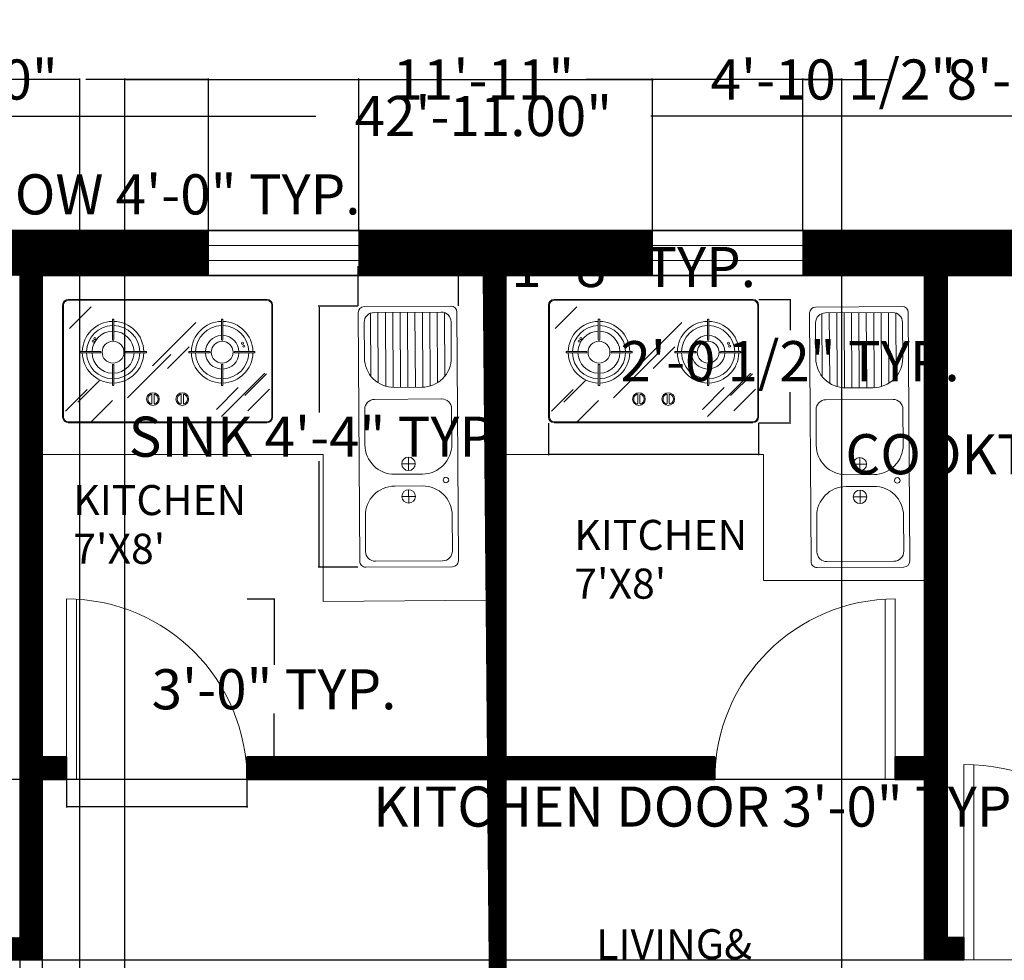
# Model space of a CAD drawing. Units: inches. Extents: x 108 to 771, y 58 to 590.
# Tile 6 of 8: x 327 to 524, y 402 to 590. Entities that reach past the tile are written whole.
import ezdxf

# ---------------------------------------------------------------- set-up
doc = ezdxf.new("R2010")
doc.units = ezdxf.units.IN
doc.header["$MEASUREMENT"] = 0
for name, color, linetype, lineweight in [('A-ANNO-DIMS', 2, 'Continuous', 13), ('A-AREA-IDEN', 7, 'Continuous', 18), ('A-DOOR', 3, 'Continuous', 18), ('A-EQPM', 9, 'Continuous', 15), ('A-FLOR-CASE', 8, 'Continuous', 18), ('A-FLOR-FIXT', 8, 'Continuous', 15), ('A-GLAZ', 4, 'Continuous', 18), ('A-WALL', 7, 'Continuous', 35), ('A-WALL-PATT', 252, 'Continuous', 9)]:
    doc.layers.add(name, color=color, linetype=linetype, lineweight=lineweight)
doc.styles.get("Standard").update_dxf_attribs({"font": 'italic8.shx'})
doc.dimstyles.get("Standard").update_dxf_attribs({"dimtxt": 8, "dimasz": 0.18, "dimexe": 0.18, "dimexo": 0.0625, "dimgap": 0.09, "dimtad": 0, "dimtih": 1, "dimtoh": 1, "dimzin": 0, "dimdsep": 46, "dimlunit": 3, "dimtxsty": 'Standard', "dimcen": 0.09, "dimclrt": 6, "dimadec": 0, "dimazin": 0, "dimtfac": 1, "dimtofl": 0, "dimtmove": 0, "dimatfit": 3, "dimfxl": 1, "dimtolj": 1, "dimtzin": 0, "dimarcsym": 0})

# ---------------------------------------------------------------- blocks, each defined once
blk = doc.blocks.new('*D5')
at = {"layer": 'A-ANNO-DIMS', "color": 0, "lineweight": -2, "transparency": 16777216}
for p, q in [((162.35, 548.12), (162.35, 571.05)), ((162.53, 570.87), (386.42, 570.87)), ((677.17, 570.87), (453.27, 570.87)), ((677.35, 548.12), (677.35, 571.05))]:
    blk.add_line(p, q, dxfattribs=at)
at = {"layer": 'A-ANNO-DIMS', "color": 0, "transparency": 16777216}
for points in [[(162.53, 570.9), (162.53, 570.84), (162.35, 570.87)], [(677.17, 570.9), (677.17, 570.84), (677.35, 570.87)]]:
    blk.add_solid(points, dxfattribs=at)
at = {"layer": 'Defpoints', "color": 0, "transparency": 16777216}
for p in [(677.35, 570.87), (162.35, 548.05), (677.35, 548.05)]:
    blk.add_point(p, dxfattribs=at)
at = {"layer": 'A-ANNO-DIMS', "color": 0, "transparency": 16777216, "insert": (419.85, 570.87), "char_height": 8, "attachment_point": 5}
blk.add_mtext('\\A1;42\'-11.00"', dxfattribs=at)
blk = doc.blocks.new('DOOR-SINGLE-39')
for p, q in [((0, 39), (0, 0)), ((2, 38.95), (2, 0)), ((0, 0), (39, 0))]:
    blk.add_line(p, q)
blk.add_arc((0, 0), 39, 0, 90)
blk = doc.blocks.new('DOOR-SINGLE-36')
for p, q in [((0, 0), (0, 36)), ((2, 0), (2, 35.94)), ((36, 0), (0, 0))]:
    blk.add_line(p, q)
blk.add_arc((0, 0), 36, 0, 90)
blk = doc.blocks.new('WINDOW-30')
for p, q in [((0, 0), (0, 30)), ((0, 30), (9, 30)), ((3, 30), (3, 0)), ((6, 30), (6, 0)), ((9, 30), (9, 0)), ((9, 0), (0, 0))]:
    blk.add_line(p, q)
blk = doc.blocks.new('COOKTOP-TWO-BURNER')
for p, q in [((40.77, 24.58), (1.12, 24.58)), ((40.77, 24.41), (1.12, 24.41)), ((0, 23.46), (0, 1.12)), ((0.17, 23.46), (0.17, 1.12)), ((1.34, 18.81), (5.66, 23.13)), ((41.72, 1.12), (41.72, 23.46)), ((41.89, 1.12), (41.89, 23.46)), ((9.92, 20.64), (10.2, 20.64)), ((9.92, 16.57), (9.92, 20.64)), ((10.2, 16.57), (10.2, 20.64)), ((17.92, 11.32), (26.57, 19.96)), ((31.97, 20.64), (31.69, 20.64)), ((31.69, 16.57), (31.69, 20.64)), ((31.97, 16.57), (31.97, 20.64)), ((7.55, 14.2), (3.53, 14.2)), ((3.53, 14.2), (3.53, 13.92)), ((7.55, 13.92), (3.53, 13.92)), ((12.57, 14.2), (16.7, 14.2)), ((12.57, 13.92), (16.7, 13.92)), ((16.7, 14.2), (16.7, 13.92)), ((20.9, 10.82), (25.22, 15.15)), ((25.19, 14.2), (25.19, 13.92)), ((29.32, 14.2), (25.19, 14.2)), ((29.32, 13.92), (25.19, 13.92)), ((34.34, 14.2), (38.36, 14.2)), ((34.34, 13.92), (38.36, 13.92)), ((38.36, 14.2), (38.36, 13.92)), ((12.96, 4.99), (21.61, 13.63)), ((9.92, 11.55), (9.92, 7.44)), ((10.2, 11.55), (10.2, 7.44)), ((31.69, 11.55), (31.69, 7.44)), ((31.7, 1.24), (40.35, 9.89)), ((31.97, 11.55), (31.97, 7.44)), ((3.04, 4.11), (7.37, 8.43)), ((36.33, 5.43), (40.66, 9.75)), ((0.56, 2.29), (4.89, 6.61)), ((9.92, 7.44), (10.2, 7.44)), ((30.71, 2.67), (35.03, 7)), ((31.97, 7.44), (31.69, 7.44)), ((36.94, 2.34), (41.26, 6.67)), ((5.63, 0.09), (9.96, 4.41)), ((17.8, 5.57), (17.8, 3.86)), ((18.24, 5.57), (18.24, 3.86)), ((23.65, 5.57), (23.65, 3.86)), ((24.09, 5.57), (24.09, 3.86)), ((1.12, 0.17), (40.77, 0.17)), ((1.12, 0), (40.77, 0))]:
    blk.add_line(p, q)
for centre, radius in [((6.11, 16.27), 0.2), ((6.44, 16.77), 0.2), ((10.06, 14.06), 2.18), ((31.83, 14.06), 2.18), ((35.9, 15.84), 0.2), ((36.13, 15.25), 0.2), ((18.02, 4.71), 1.26), ((23.87, 4.71), 1.26)]:
    blk.add_circle(centre, radius)
for centre, radius, start, end in [((1.12, 23.46), 1.12, 90, 180), ((1.12, 23.46), 0.95, 90, 180), ((40.77, 23.46), 1.12, 0, 90), ((40.77, 23.46), 0.95, 0, 90), ((10.06, 14.06), 6.14, 91.3023, 178.6977), ((10.06, 14.06), 6.14, 1.3023, 88.6977), ((31.83, 14.06), 6.14, 91.3023, 178.6977), ((31.83, 14.06), 6.14, 1.3023, 88.6977), ((10.06, 14.06), 5.31, 91.5918, 178.4082), ((10.06, 14.06), 4.19, 91.9102, 178.0898), ((10.06, 14.06), 4.19, 1.9102, 88.0898), ((10.06, 14.06), 5.31, 1.5918, 88.4082), ((31.83, 14.06), 5.31, 91.5918, 178.4082), ((31.83, 14.06), 5.31, 1.5918, 88.4082), ((10.06, 16.59), 0.141, 186.7354, 353.2646), ((31.83, 14.06), 3.35, 92.388, 177.612), ((31.83, 16.58), 0.14, 183.9579, 356.0421), ((31.83, 14.06), 3.35, 2.388, 87.612), ((10.06, 14.06), 6.14, 181.3023, 268.6977), ((10.06, 14.06), 5.31, 181.5918, 268.4082), ((10.06, 14.06), 4.19, 181.9102, 268.0898), ((7.5, 14.06), 0.147, 288.751, 71.249), ((10.06, 14.06), 4.19, 271.9102, 358.0898), ((10.06, 14.06), 6.14, 271.3023, 358.6977), ((10.06, 14.06), 5.31, 271.5918, 358.4082), ((12.62, 14.06), 0.149, 110.5507, 249.4493), ((31.83, 14.06), 6.14, 181.3023, 268.6977), ((31.83, 14.06), 5.31, 181.5918, 268.4082), ((31.83, 14.06), 3.35, 182.388, 267.612), ((29.28, 14.06), 0.147, 288.412, 71.588), ((31.83, 14.06), 3.35, 272.388, 357.612), ((31.83, 14.06), 6.14, 271.3023, 358.6977), ((31.83, 14.06), 5.31, 271.5918, 358.4082), ((34.38, 14.06), 0.144, 104.2945, 255.7055), ((10.06, 11.49), 0.15, 21.7885, 158.2115), ((31.83, 11.51), 0.147, 17.9418, 162.0582), ((18.02, 4.71), 1.03, 111.3237, 248.6763), ((17.69, 5.57), 0.112, 0, 111.3237), ((18.36, 5.57), 0.112, 68.6763, 180), ((18.02, 4.71), 1.03, 291.3237, 68.6763), ((23.87, 4.71), 1.03, 111.3237, 248.6763), ((23.53, 5.57), 0.112, 0, 111.3237), ((24.2, 5.57), 0.112, 68.6763, 180), ((23.87, 4.71), 1.03, 291.3237, 68.6763), ((17.69, 3.86), 0.112, 248.6763, 0), ((18.36, 3.86), 0.112, 180, 291.3237), ((23.53, 3.86), 0.112, 248.6763, 0), ((24.2, 3.86), 0.112, 180, 291.3237), ((1.12, 1.12), 1.12, 180, 270), ((1.12, 1.12), 0.95, 180, 270), ((40.77, 1.12), 0.95, 270, 360), ((40.77, 1.12), 1.12, 270, 360)]:
    blk.add_arc(centre, radius, start, end)
blk = doc.blocks.new('SINK-DOUBLE-DRAINBOARD')
for p, q in [((18.5, 52.07), (1.17, 51.97)), ((0, 50.78), (0.28, 1.17)), ((2.44, 50.65), (2.52, 38.11)), ((16.54, 50.87), (3.15, 50.8)), ((3.92, 50.8), (4, 36.77)), ((5.4, 50.81), (5.48, 36.1)), ((6.87, 50.82), (6.96, 35.86)), ((8.35, 50.83), (8.43, 35.87)), ((9.82, 50.84), (9.91, 35.88)), ((11.3, 50.84), (11.39, 35.88)), ((12.78, 50.85), (12.86, 35.89)), ((14.25, 50.86), (14.34, 36.13)), ((15.73, 50.87), (15.81, 36.8)), ((17.21, 50.77), (17.28, 38.11)), ((19.68, 50.89), (19.97, 1.29)), ((1.23, 41.73), (1.19, 48.82)), ((18.56, 41.83), (18.52, 48.92)), ((12.68, 35.89), (7.17, 35.86)), ((16.63, 33.55), (3.25, 33.48)), ((1.33, 24.41), (1.29, 31.5)), ((18.66, 24.51), (18.61, 31.59)), ((10.02, 19.28), (10.01, 21.96)), ((11.36, 20.63), (8.67, 20.62)), ((12.78, 18.57), (7.27, 18.54)), ((12.8, 16.21), (7.29, 16.18)), ((11.39, 14.13), (8.71, 14.11)), ((10.06, 12.78), (10.05, 15.46)), ((1.41, 10.24), (1.45, 3.15)), ((18.74, 10.34), (18.78, 3.25)), ((18.8, 0.1), (1.47, 0)), ((16.82, 1.27), (3.43, 1.19))]:
    blk.add_line(p, q)
for centre, radius in [((10.02, 20.62), 1.34), ((17.48, 17.39), 0.554), ((10.05, 14.12), 1.34)]:
    blk.add_circle(centre, radius)
for centre, radius, start, end in [((1.18, 50.79), 1.18, 90.3287, 180.3287), ((18.5, 50.89), 1.18, 0.3287, 90.3287), ((3.16, 48.83), 1.97, 90.3287, 180.3287), ((16.55, 48.91), 1.97, 0.3287, 90.3287), ((7.14, 41.77), 5.91, 180.3287, 270.3287), ((12.65, 41.8), 5.91, 270.3287, 0.3287), ((3.26, 31.51), 1.97, 90.3287, 180.3287), ((16.65, 31.58), 1.97, 0.3287, 90.3287), ((7.24, 24.44), 5.91, 180.3287, 270.3287), ((12.75, 24.47), 5.91, 270.3287, 0.3287), ((7.32, 10.27), 5.91, 90.3287, 180.3287), ((12.83, 10.3), 5.91, 0.3287, 90.3287), ((3.42, 3.16), 1.97, 180.3287, 270.3287), ((16.81, 3.24), 1.97, 270.3287, 0.3287), ((1.47, 1.18), 1.18, 180.3287, 270.3287), ((18.79, 1.28), 1.18, 270.3287, 0.3287)]:
    blk.add_arc(centre, radius, start, end)
blk = doc.blocks.new('*D20')
at = {"layer": 'A-ANNO-DIMS', "color": 0, "lineweight": -2, "transparency": 16777216}
for p, q in [((232.77, 548.12), (232.77, 555.43)), ((232.95, 555.25), (280.59, 555.25)), ((280.77, 548.12), (280.77, 555.43)), ((280.77, 555.25), (280.95, 555.25))]:
    blk.add_line(p, q, dxfattribs=at)
at = {"layer": 'A-ANNO-DIMS', "color": 0, "transparency": 16777216}
for points in [[(232.95, 555.28), (232.95, 555.22), (232.77, 555.25)], [(280.59, 555.28), (280.59, 555.22), (280.77, 555.25)]]:
    blk.add_solid(points, dxfattribs=at)
at = {"layer": 'Defpoints', "color": 0, "transparency": 16777216}
for p in [(280.77, 555.25), (232.77, 548.05), (280.77, 548.05)]:
    blk.add_point(p, dxfattribs=at)
at = {"layer": 'A-ANNO-DIMS', "color": 6, "transparency": 16777216, "insert": (346.76, 555.25), "char_height": 8, "attachment_point": 5}
blk.add_mtext('\\A1;WINDOW 4\'-0" TYP.', dxfattribs=at)
blk = doc.blocks.new('*D26')
at = {"layer": 'A-ANNO-DIMS', "color": 0, "lineweight": -2, "transparency": 16777216}
for p, q in [((336.68, 438.49), (336.68, 432.97)), ((372.68, 438.49), (372.68, 432.97)), ((336.86, 433.15), (372.5, 433.15)), ((372.68, 433.15), (372.86, 433.15))]:
    blk.add_line(p, q, dxfattribs=at)
at = {"layer": 'A-ANNO-DIMS', "color": 0, "transparency": 16777216}
for points in [[(336.86, 433.18), (336.86, 433.12), (336.68, 433.15)], [(372.5, 433.18), (372.5, 433.12), (372.68, 433.15)]]:
    blk.add_solid(points, dxfattribs=at)
at = {"layer": 'Defpoints', "color": 0, "transparency": 16777216}
for p in [(336.68, 438.55), (372.68, 438.55), (372.68, 433.15)]:
    blk.add_point(p, dxfattribs=at)
at = {"layer": 'A-ANNO-DIMS', "color": 6, "transparency": 16777216, "insert": (463.04, 433.15), "char_height": 8, "attachment_point": 5}
blk.add_mtext('\\A1;KITCHEN DOOR 3\'-0" TYP.', dxfattribs=at)
blk = doc.blocks.new('*D27')
at = {"layer": 'A-ANNO-DIMS', "color": 0, "lineweight": -2, "transparency": 16777216}
for p, q in [((372.74, 474.55), (378.26, 474.55)), ((378.08, 474.37), (378.08, 461.41)), ((378.08, 438.73), (378.08, 451.7)), ((372.74, 438.55), (378.26, 438.55))]:
    blk.add_line(p, q, dxfattribs=at)
at = {"layer": 'A-ANNO-DIMS', "color": 0, "transparency": 16777216}
for points in [[(378.05, 474.37), (378.11, 474.37), (378.08, 474.55)], [(378.05, 438.73), (378.11, 438.73), (378.08, 438.55)]]:
    blk.add_solid(points, dxfattribs=at)
at = {"layer": 'Defpoints', "color": 0, "transparency": 16777216}
for p in [(372.68, 474.55), (378.08, 474.55), (372.68, 438.55)]:
    blk.add_point(p, dxfattribs=at)
at = {"layer": 'A-ANNO-DIMS', "color": 6, "transparency": 16777216, "insert": (378.08, 456.55), "char_height": 8, "attachment_point": 5}
blk.add_mtext('\\A1;3\'-0" TYP.', dxfattribs=at)
blk = doc.blocks.new('*D38')
at = {"layer": 'A-ANNO-DIMS', "color": 0, "lineweight": -2, "transparency": 16777216}
for p, q in [((606.93, 385.95), (606.93, 394.93)), ((665.98, 385.95), (665.98, 394.93)), ((606.93, 394.75), (606.75, 394.75)), ((665.8, 394.75), (607.11, 394.75))]:
    blk.add_line(p, q, dxfattribs=at)
at = {"layer": 'A-ANNO-DIMS', "color": 0, "transparency": 16777216}
for points in [[(607.11, 394.78), (607.11, 394.72), (606.93, 394.75)], [(665.8, 394.78), (665.8, 394.72), (665.98, 394.75)]]:
    blk.add_solid(points, dxfattribs=at)
at = {"layer": 'Defpoints', "color": 0, "transparency": 16777216}
for p in [(606.93, 394.75), (606.93, 385.89), (665.98, 385.89)]:
    blk.add_point(p, dxfattribs=at)
at = {"layer": 'A-ANNO-DIMS', "color": 6, "transparency": 16777216, "insert": (552.56, 394.75), "char_height": 8, "attachment_point": 5}
blk.add_mtext('\\A1;TUB 4\'-11" TYP.', dxfattribs=at)
blk = doc.blocks.new('*D40')
at = {"layer": 'A-ANNO-DIMS', "color": 0, "lineweight": -2, "transparency": 16777216}
for p, q in [((432.85, 509.64), (432.85, 503.24)), ((474.74, 509.64), (474.74, 503.24)), ((433.03, 503.42), (474.56, 503.42)), ((474.74, 503.42), (474.92, 503.42))]:
    blk.add_line(p, q, dxfattribs=at)
at = {"layer": 'A-ANNO-DIMS', "color": 0, "transparency": 16777216}
for points in [[(433.03, 503.45), (433.03, 503.39), (432.85, 503.42)], [(474.56, 503.45), (474.56, 503.39), (474.74, 503.42)]]:
    blk.add_solid(points, dxfattribs=at)
at = {"layer": 'Defpoints', "color": 0, "transparency": 16777216}
for p in [(432.85, 509.7), (474.74, 509.7), (474.74, 503.42)]:
    blk.add_point(p, dxfattribs=at)
at = {"layer": 'A-ANNO-DIMS', "color": 6, "transparency": 16777216, "insert": (543.58, 503.42), "char_height": 8, "attachment_point": 5}
blk.add_mtext('\\A1;COOKTOP 3\'-6" TYP.', dxfattribs=at)
blk = doc.blocks.new('*D41')
at = {"layer": 'A-ANNO-DIMS', "color": 0, "lineweight": -2, "transparency": 16777216}
for p, q in [((474.8, 534.28), (481.2, 534.28)), ((481.02, 534.1), (481.02, 528.18)), ((481.02, 509.88), (481.02, 515.81)), ((474.8, 509.7), (481.2, 509.7))]:
    blk.add_line(p, q, dxfattribs=at)
at = {"layer": 'A-ANNO-DIMS', "color": 0, "transparency": 16777216}
for points in [[(480.99, 534.1), (481.05, 534.1), (481.02, 534.28)], [(480.99, 509.88), (481.05, 509.88), (481.02, 509.7)]]:
    blk.add_solid(points, dxfattribs=at)
at = {"layer": 'Defpoints', "color": 0, "transparency": 16777216}
for p in [(474.74, 534.28), (481.02, 534.28), (474.74, 509.7)]:
    blk.add_point(p, dxfattribs=at)
at = {"layer": 'A-ANNO-DIMS', "color": 6, "transparency": 16777216, "insert": (481.02, 521.99), "char_height": 8, "attachment_point": 5}
blk.add_mtext('\\A1;2\'-0 1/2" TYP.', dxfattribs=at)
blk = doc.blocks.new('*D42')
at = {"layer": 'A-ANNO-DIMS', "color": 0, "lineweight": -2, "transparency": 16777216}
for p, q in [((394.82, 532.96), (386.89, 532.96)), ((387.07, 532.78), (387.07, 511.77)), ((387.07, 481.07), (387.07, 502.07)), ((394.82, 480.89), (386.89, 480.89))]:
    blk.add_line(p, q, dxfattribs=at)
at = {"layer": 'A-ANNO-DIMS', "color": 0, "transparency": 16777216}
for points in [[(387.04, 532.78), (387.1, 532.78), (387.07, 532.96)], [(387.04, 481.07), (387.1, 481.07), (387.07, 480.89)]]:
    blk.add_solid(points, dxfattribs=at)
at = {"layer": 'Defpoints', "color": 0, "transparency": 16777216}
for p in [(387.07, 532.96), (394.88, 532.96), (394.88, 480.89)]:
    blk.add_point(p, dxfattribs=at)
at = {"layer": 'A-ANNO-DIMS', "color": 6, "transparency": 16777216, "insert": (387.07, 506.92), "char_height": 8, "attachment_point": 5}
blk.add_mtext('\\A1;SINK 4\'-4" TYP.', dxfattribs=at)
blk = doc.blocks.new('*D43')
at = {"layer": 'A-ANNO-DIMS', "color": 0, "lineweight": -2, "transparency": 16777216}
for p, q in [((394.88, 533.02), (394.88, 540.95)), ((395.06, 540.77), (414.68, 540.77)), ((414.86, 533.02), (414.86, 540.95)), ((414.86, 540.77), (415.04, 540.77))]:
    blk.add_line(p, q, dxfattribs=at)
at = {"layer": 'A-ANNO-DIMS', "color": 0, "transparency": 16777216}
for points in [[(395.06, 540.8), (395.06, 540.74), (394.88, 540.77)], [(414.68, 540.8), (414.68, 540.74), (414.86, 540.77)]]:
    blk.add_solid(points, dxfattribs=at)
at = {"layer": 'Defpoints', "color": 0, "transparency": 16777216}
for p in [(414.86, 540.77), (394.88, 532.96), (414.86, 532.96)]:
    blk.add_point(p, dxfattribs=at)
at = {"layer": 'A-ANNO-DIMS', "color": 6, "transparency": 16777216, "insert": (449.8, 540.77), "char_height": 8, "attachment_point": 5}
blk.add_mtext('\\A1;1\'-8" TYP.', dxfattribs=at)
blk = doc.blocks.new('*D52')
at = {"layer": 'A-ANNO-DIMS', "color": 0, "lineweight": -2, "transparency": 16777216}
for p, q in [((348.35, 145.12), (348.35, 578.33)), ((348.53, 578.15), (399.37, 578.15)), ((491.17, 578.15), (440.32, 578.15)), ((491.35, 145.12), (491.35, 578.33))]:
    blk.add_line(p, q, dxfattribs=at)
at = {"layer": 'A-ANNO-DIMS', "color": 0, "transparency": 16777216}
for points in [[(348.53, 578.18), (348.53, 578.12), (348.35, 578.15)], [(491.17, 578.18), (491.17, 578.12), (491.35, 578.15)]]:
    blk.add_solid(points, dxfattribs=at)
at = {"layer": 'Defpoints', "color": 0, "transparency": 16777216}
for p in [(491.35, 578.15), (348.35, 145.05), (491.35, 145.05)]:
    blk.add_point(p, dxfattribs=at)
at = {"layer": 'A-ANNO-DIMS', "color": 6, "transparency": 16777216, "insert": (419.85, 578.15), "char_height": 8, "attachment_point": 5}
blk.add_mtext('\\A1;11\'-11"', dxfattribs=at)
blk = doc.blocks.new('*D54')
at = {"layer": 'A-ANNO-DIMS', "color": 0, "lineweight": -2, "transparency": 16777216}
for p, q in [((280.77, 548.12), (280.77, 578.33)), ((280.95, 578.15), (305.28, 578.15)), ((364.84, 578.15), (340.51, 578.15)), ((365.02, 548.12), (365.02, 578.33))]:
    blk.add_line(p, q, dxfattribs=at)
at = {"layer": 'A-ANNO-DIMS', "color": 0, "transparency": 16777216}
for points in [[(280.95, 578.18), (280.95, 578.12), (280.77, 578.15)], [(364.84, 578.18), (364.84, 578.12), (365.02, 578.15)]]:
    blk.add_solid(points, dxfattribs=at)
at = {"layer": 'Defpoints', "color": 0, "transparency": 16777216}
for p in [(365.02, 578.15), (280.77, 548.05), (365.02, 548.05)]:
    blk.add_point(p, dxfattribs=at)
at = {"layer": 'A-ANNO-DIMS', "color": 6, "transparency": 16777216, "insert": (322.9, 578.15), "char_height": 8, "attachment_point": 5}
blk.add_mtext('\\A1;7\'-0"', dxfattribs=at)
blk = doc.blocks.new('*D55')
at = {"layer": 'A-ANNO-DIMS', "color": 0, "lineweight": -2, "transparency": 16777216}
for p, q in [((395.02, 548.12), (395.02, 578.33)), ((395.2, 578.15), (453.4, 578.15)), ((453.58, 548.12), (453.58, 578.33)), ((453.58, 578.15), (453.76, 578.15))]:
    blk.add_line(p, q, dxfattribs=at)
at = {"layer": 'A-ANNO-DIMS', "color": 0, "transparency": 16777216}
for points in [[(395.2, 578.18), (395.2, 578.12), (395.02, 578.15)], [(453.4, 578.18), (453.4, 578.12), (453.58, 578.15)]]:
    blk.add_solid(points, dxfattribs=at)
at = {"layer": 'Defpoints', "color": 0, "transparency": 16777216}
for p in [(453.58, 578.15), (395.02, 548.05), (453.58, 548.05)]:
    blk.add_point(p, dxfattribs=at)
at = {"layer": 'A-ANNO-DIMS', "color": 6, "transparency": 16777216, "insert": (489.66, 578.15), "char_height": 8, "attachment_point": 5}
blk.add_mtext('\\A1;4\'-10 1/2"', dxfattribs=at)
blk = doc.blocks.new('*D56')
at = {"layer": 'A-ANNO-DIMS', "color": 0, "lineweight": -2, "transparency": 16777216}
for p, q in [((483.58, 548.12), (483.58, 578.33)), ((483.76, 578.15), (500.52, 578.15)), ((583.74, 578.15), (566.98, 578.15)), ((583.92, 548.12), (583.92, 578.33))]:
    blk.add_line(p, q, dxfattribs=at)
at = {"layer": 'A-ANNO-DIMS', "color": 0, "transparency": 16777216}
for points in [[(483.76, 578.18), (483.76, 578.12), (483.58, 578.15)], [(583.74, 578.18), (583.74, 578.12), (583.92, 578.15)]]:
    blk.add_solid(points, dxfattribs=at)
at = {"layer": 'Defpoints', "color": 0, "transparency": 16777216}
for p in [(583.92, 578.15), (483.58, 548.05), (583.92, 548.05)]:
    blk.add_point(p, dxfattribs=at)
at = {"layer": 'A-ANNO-DIMS', "color": 6, "transparency": 16777216, "insert": (533.75, 578.15), "char_height": 8, "attachment_point": 5}
blk.add_mtext('\\A1;8\'-4 1/2"', dxfattribs=at)
blk = doc.blocks.new('*D59')
at = {"layer": 'A-ANNO-DIMS', "color": 0, "lineweight": -2, "transparency": 16777216}
for p, q in [((327.35, 538.99), (327.35, 69.77)), ((331.85, 538.99), (331.85, 69.77)), ((327.53, 69.95), (331.67, 69.95)), ((331.85, 69.95), (332.03, 69.95))]:
    blk.add_line(p, q, dxfattribs=at)
at = {"layer": 'A-ANNO-DIMS', "color": 0, "transparency": 16777216}
for points in [[(327.53, 69.98), (327.53, 69.92), (327.35, 69.95)], [(331.67, 69.98), (331.67, 69.92), (331.85, 69.95)]]:
    blk.add_solid(points, dxfattribs=at)
at = {"layer": 'Defpoints', "color": 0, "transparency": 16777216}
for p in [(327.35, 539.05), (331.85, 539.05), (331.85, 69.95)]:
    blk.add_point(p, dxfattribs=at)
at = {"layer": 'A-ANNO-DIMS', "color": 6, "transparency": 16777216, "insert": (365.26, 69.95), "char_height": 8, "attachment_point": 5}
blk.add_mtext('\\A1;0\'-4 1/2"', dxfattribs=at)
blk = doc.blocks.new('*D60')
at = {"layer": 'A-ANNO-DIMS', "color": 0, "lineweight": -2, "transparency": 16777216}
for p, q in [((171.35, 145.12), (171.35, 578.33)), ((171.53, 578.15), (234.87, 578.15)), ((339.17, 578.15), (275.82, 578.15)), ((339.35, 145.12), (339.35, 578.33))]:
    blk.add_line(p, q, dxfattribs=at)
at = {"layer": 'A-ANNO-DIMS', "color": 0, "transparency": 16777216}
for points in [[(171.53, 578.18), (171.53, 578.12), (171.35, 578.15)], [(339.17, 578.18), (339.17, 578.12), (339.35, 578.15)]]:
    blk.add_solid(points, dxfattribs=at)
at = {"layer": 'Defpoints', "color": 0, "transparency": 16777216}
for p in [(339.35, 578.15), (171.35, 145.05), (339.35, 145.05)]:
    blk.add_point(p, dxfattribs=at)
at = {"layer": 'A-ANNO-DIMS', "color": 6, "transparency": 16777216, "insert": (255.35, 578.15), "char_height": 8, "attachment_point": 5}
blk.add_mtext('\\A1;14\'-0"', dxfattribs=at)
blk = doc.blocks.new('*D62')
at = {"layer": 'A-ANNO-DIMS', "color": 0, "lineweight": -2, "transparency": 16777216}
for p, q in [((507.78, 438.55), (132.07, 438.55)), ((132.25, 438.37), (132.25, 425.4)), ((132.25, 402.73), (132.25, 415.7)), ((515.6, 402.55), (132.07, 402.55))]:
    blk.add_line(p, q, dxfattribs=at)
at = {"layer": 'A-ANNO-DIMS', "color": 0, "transparency": 16777216}
for points in [[(132.22, 438.37), (132.28, 438.37), (132.25, 438.55)], [(132.22, 402.73), (132.28, 402.73), (132.25, 402.55)]]:
    blk.add_solid(points, dxfattribs=at)
at = {"layer": 'Defpoints', "color": 0, "transparency": 16777216}
for p in [(507.85, 438.55), (132.25, 402.55), (515.66, 402.55)]:
    blk.add_point(p, dxfattribs=at)
at = {"layer": 'A-ANNO-DIMS', "color": 6, "transparency": 16777216, "insert": (132.25, 420.55), "char_height": 8, "attachment_point": 5}
blk.add_mtext('\\A1;3\'-0"', dxfattribs=at)

msp = doc.modelspace()

# ---------------------------------------------------------------- hatches: boundary and pattern name
at = {"layer": 'A-WALL-PATT'}
h = msp.add_hatch(dxfattribs=at)
h.set_pattern_fill('ANSI31', color=256)
h.paths.add_polyline_path([(171.345, 461.548), (162.345, 461.548), (162.345, 390.901), (171.345, 390.901), (171.345, 393.51), (171.345, 402.553), (233.142, 402.553), (233.142, 407.053), (171.345, 407.053)])
h.paths.add_polyline_path([(331.845, 438.553), (336.68, 438.554), (336.68, 443.053), (331.845, 443.053), (331.845, 539.053), (365.02, 539.053), (365.02, 548.053), (280.772, 548.053), (280.772, 539.053), (327.345, 539.053), (327.345, 407.053), (325.63, 407.053), (325.63, 402.553), (331.845, 402.553)])
h.paths.add_polyline_path([(286.63, 407.053), (263.142, 407.053), (263.142, 402.553), (267.345, 402.553), (267.345, 352.303), (171.345, 352.303), (171.345, 360.901), (162.345, 360.901), (162.345, 336.026), (171.345, 336.026), (171.345, 347.803), (267.345, 347.803), (267.345, 293.053), (263.142, 293.053), (263.142, 288.553), (293.037, 288.553), (293.037, 293.053), (271.845, 293.053), (271.845, 402.553), (286.63, 402.553)])
h.paths.add_polyline_path([(466.018, 443.053), (424.345, 443.053), (424.345, 539.053), (453.584, 539.053), (453.584, 548.053), (395.02, 548.053), (395.02, 539.053), (419.845, 539.053), (420.71, 443.053), (372.68, 443.053), (372.68, 438.557), (420.751, 438.561), (421.075, 402.553), (422.061, 293.053), (419.994, 293.053), (419.994, 288.553), (426.124, 288.553), (426.124, 293.053), (424.345, 293.053), (424.345, 402.553), (424.345, 438.553), (466.018, 438.553)])
h.paths.add_polyline_path([(512.345, 539.053), (583.918, 539.053), (583.918, 548.053), (483.584, 548.053), (483.584, 539.053), (507.845, 539.053), (507.845, 443.053), (502.018, 443.053), (502.018, 438.553), (507.845, 438.553), (507.845, 402.553), (515.658, 402.553), (515.658, 407.053), (512.345, 407.053)])
h.paths.add_polyline_path([(232.772, 548.053), (162.345, 548.053), (162.345, 509.548), (171.345, 509.548), (171.345, 539.053), (232.772, 539.053)])
h.paths.add_polyline_path([(233.142, 293.053), (171.345, 293.053), (171.345, 306.026), (162.345, 306.026), (162.345, 230.8), (171.345, 230.8), (171.345, 288.553), (233.142, 288.553)])
h.paths.add_polyline_path([(359.994, 293.053), (332.037, 293.053), (332.037, 288.553), (339.345, 288.553), (339.345, 145.053), (334.469, 145.053), (334.469, 136.053), (339.345, 136.053), (339.345, 104.553), (166.845, 104.553), (166.845, 136.053), (211.837, 136.053), (211.837, 145.053), (171.345, 145.053), (171.345, 182.8), (162.345, 182.8), (162.345, 100.053), (343.845, 100.053), (343.845, 136.053), (400.886, 136.053), (400.886, 145.053), (348.345, 145.053), (348.345, 288.553), (359.994, 288.553)])
h.paths.add_polyline_path([(500.345, 288.553), (503.755, 288.553), (503.755, 293.053), (486.124, 293.053), (486.124, 288.553), (491.345, 288.553), (491.345, 145.053), (448.886, 145.053), (448.886, 136.053), (495.845, 136.053), (495.845, 100.053), (677.345, 100.053), (677.345, 186.265), (668.345, 186.265), (668.345, 145.053), (627.637, 145.053), (627.637, 136.053), (672.845, 136.053), (672.845, 104.278), (500.345, 104.539), (500.345, 136.053), (504.239, 136.053), (504.239, 145.053), (500.345, 145.053)])
h.paths.add_polyline_path([(580.913, 293.053), (572.345, 293.053), (572.345, 347.803), (668.345, 347.803), (668.345, 330.831), (677.345, 330.831), (677.345, 366.853), (668.345, 366.853), (668.345, 352.303), (572.345, 352.303), (572.345, 402.553), (580.418, 402.553), (580.418, 407.053), (554.658, 407.053), (554.658, 402.553), (567.845, 402.553), (567.845, 293.053), (542.755, 293.053), (542.755, 288.553), (580.913, 288.553)])
h.paths.add_polyline_path([(677.345, 300.831), (668.345, 300.831), (668.345, 293.053), (610.913, 293.053), (610.913, 288.553), (668.345, 288.553), (668.345, 234.265), (677.345, 234.265)])
h.paths.add_polyline_path([(304.469, 145.053), (259.837, 145.053), (259.837, 136.053), (304.469, 136.053)], flags=17)
h.paths.add_polyline_path([(579.637, 145.053), (534.239, 145.053), (534.239, 136.053), (579.637, 136.053)], flags=17)
h.paths.add_polyline_path([(677.345, 450.416), (668.345, 450.416), (668.345, 407.053), (610.418, 407.053), (610.418, 402.553), (668.345, 402.553), (668.345, 396.853), (677.345, 396.853)])
h.paths.add_polyline_path([(677.345, 548.053), (631.918, 548.053), (631.918, 539.053), (668.345, 539.053), (668.345, 498.416), (677.345, 498.416)])
h = msp.add_hatch(dxfattribs=at)
h.set_pattern_fill('ANSI31', color=256)
h.paths.add_polyline_path([(365.02, 548.053), (280.772, 548.053), (280.772, 539.053), (327.345, 539.053), (327.345, 407.053), (325.63, 407.053), (325.63, 402.553), (331.845, 402.553), (331.845, 438.553), (336.68, 438.554), (336.68, 443.053), (331.845, 443.053), (331.845, 539.053), (365.02, 539.053)])
h.paths.add_polyline_path([(453.584, 548.053), (395.02, 548.053), (395.02, 539.053), (419.845, 539.053), (420.71, 443.053), (372.68, 443.053), (372.68, 438.557), (420.751, 438.561), (421.075, 402.553), (422.061, 293.053), (419.994, 293.053), (419.994, 288.553), (426.124, 288.553), (426.124, 293.053), (424.345, 293.053), (424.345, 402.553), (424.345, 438.553), (466.018, 438.553), (466.018, 443.053), (424.345, 443.053), (424.345, 539.053), (453.584, 539.053)])
h.paths.add_polyline_path([(232.772, 548.053), (162.345, 548.053), (162.345, 509.548), (171.345, 509.548), (171.345, 539.053), (232.772, 539.053)])
h.paths.add_polyline_path([(171.345, 461.548), (162.345, 461.548), (162.345, 390.901), (171.345, 390.901), (171.345, 393.51), (171.345, 402.553), (233.142, 402.553), (233.142, 407.053), (171.345, 407.053)])
h.paths.add_polyline_path([(286.63, 407.053), (263.142, 407.053), (263.142, 402.553), (267.345, 402.553), (267.345, 352.303), (171.345, 352.303), (171.345, 360.901), (162.345, 360.901), (162.345, 336.026), (171.345, 336.026), (171.345, 347.803), (267.345, 347.803), (267.345, 293.053), (263.142, 293.053), (263.142, 288.553), (293.037, 288.553), (293.037, 293.053), (271.845, 293.053), (271.845, 402.553), (286.63, 402.553)])
h.paths.add_polyline_path([(171.345, 306.026), (162.345, 306.026), (162.345, 230.8), (171.345, 230.8), (171.345, 288.553), (233.142, 288.553), (233.142, 293.053), (171.345, 293.053)])
h.paths.add_polyline_path([(348.345, 288.553), (359.994, 288.553), (359.994, 293.053), (332.037, 293.053), (332.037, 288.553), (339.345, 288.553), (339.345, 145.053), (334.469, 145.053), (334.469, 136.053), (339.345, 136.053), (339.345, 104.553), (166.845, 104.553), (166.845, 136.053), (211.837, 136.053), (211.837, 145.053), (171.345, 145.053), (171.345, 182.8), (162.345, 182.8), (162.345, 100.053), (343.845, 100.053), (343.845, 136.053), (400.886, 136.053), (400.886, 145.053), (348.345, 145.053)])
h.paths.add_polyline_path([(503.755, 293.053), (486.124, 293.053), (486.124, 288.553), (491.345, 288.553), (491.345, 145.053), (448.886, 145.053), (448.886, 136.053), (495.845, 136.053), (495.845, 100.053), (677.345, 100.053), (677.345, 186.265), (668.345, 186.265), (668.345, 145.053), (627.637, 145.053), (627.637, 136.053), (672.845, 136.053), (672.845, 104.278), (500.345, 104.539), (500.345, 136.053), (504.239, 136.053), (504.239, 145.053), (500.345, 145.053), (500.345, 288.553), (503.755, 288.553)])
h.paths.add_polyline_path([(580.913, 293.053), (572.345, 293.053), (572.345, 347.803), (668.345, 347.803), (668.345, 330.831), (677.345, 330.831), (677.345, 366.853), (668.345, 366.853), (668.345, 352.303), (572.345, 352.303), (572.345, 402.553), (580.418, 402.553), (580.418, 407.053), (554.658, 407.053), (554.658, 402.553), (567.845, 402.553), (567.845, 293.053), (542.755, 293.053), (542.755, 288.553), (580.913, 288.553)])
h.paths.add_polyline_path([(677.345, 300.831), (668.345, 300.831), (668.345, 293.053), (610.913, 293.053), (610.913, 288.553), (668.345, 288.553), (668.345, 234.265), (677.345, 234.265)])
h.paths.add_polyline_path([(579.637, 145.053), (534.239, 145.053), (534.239, 136.053), (579.637, 136.053)], flags=17)
h.paths.add_polyline_path([(304.469, 145.053), (259.837, 145.053), (259.837, 136.053), (304.469, 136.053)], flags=17)
h.paths.add_polyline_path([(583.918, 548.053), (483.584, 548.053), (483.584, 539.053), (507.845, 539.053), (507.845, 443.053), (502.018, 443.053), (502.018, 438.553), (507.845, 438.553), (507.845, 402.553), (515.658, 402.553), (515.658, 407.053), (512.345, 407.053), (512.345, 539.053), (583.918, 539.053)])
h.paths.add_polyline_path([(677.345, 548.053), (631.918, 548.053), (631.918, 539.053), (668.345, 539.053), (668.345, 498.416), (677.345, 498.416)])
h.paths.add_polyline_path([(677.345, 450.416), (668.345, 450.416), (668.345, 407.053), (610.418, 407.053), (610.418, 402.553), (668.345, 402.553), (668.345, 396.853), (677.345, 396.853)])

# ---------------------------------------------------------------- linework, layer by layer
at = {"layer": 'A-FLOR-CASE'}
for p, q in [((331.845, 503.364), (387.855, 503.364)), ((387.855, 503.364), (387.855, 474.038)), ((424.345, 503.364), (475.728, 503.364)), ((475.728, 503.364), (475.728, 478.253)), ((475.728, 478.253), (507.845, 478.253)), ((387.855, 474.038), (420.428, 474.332))]:
    msp.add_line(p, q, dxfattribs=at)
at = {"layer": 'A-WALL'}
for p, q in [((162.345, 548.053), (677.345, 548.053)), ((331.845, 539.053), (419.845, 539.053)), ((331.845, 443.053), (331.845, 539.053)), ((420.71, 443.053), (419.845, 539.053)), ((424.345, 539.053), (507.845, 539.053)), ((424.345, 443.053), (424.345, 539.053)), ((507.845, 539.053), (507.845, 443.053)), ((512.345, 539.053), (512.345, 407.053)), ((512.345, 539.053), (668.345, 539.053)), ((331.845, 443.053), (336.68, 443.053)), ((336.68, 438.554), (336.68, 443.053)), ((372.68, 438.554), (372.68, 443.053)), ((372.68, 443.053), (420.71, 443.053)), ((424.345, 443.053), (466.018, 443.053)), ((466.018, 438.553), (466.018, 443.053)), ((502.018, 438.553), (502.018, 443.053)), ((502.018, 443.053), (507.845, 443.053)), ((331.845, 438.553), (336.68, 438.554)), ((331.845, 402.553), (331.845, 438.553)), ((372.68, 438.557), (420.751, 438.561)), ((421.075, 402.553), (420.751, 438.561)), ((424.345, 402.553), (424.345, 438.553)), ((424.345, 438.553), (466.018, 438.553)), ((502.018, 438.553), (507.845, 438.553)), ((507.845, 438.553), (507.845, 402.553)), ((512.345, 407.053), (515.658, 407.053)), ((515.658, 407.053), (515.658, 402.553)), ((325.63, 402.553), (331.845, 402.553)), ((422.061, 293.053), (421.075, 402.553)), ((424.345, 293.053), (424.345, 402.553)), ((507.845, 402.553), (515.658, 402.553))]:
    msp.add_line(p, q, dxfattribs=at)

# ---------------------------------------------------------------- block references
at = {"layer": 'A-DOOR'}
for name, p in [('DOOR-SINGLE-36', (336.68, 438.554)), ('DOOR-SINGLE-39', (515.658, 402.553))]:
    msp.add_blockref(name, p, dxfattribs=at)
at = {"layer": 'A-DOOR', "extrusion": (0, 0, -1), "zscale": -1}
msp.add_blockref('DOOR-SINGLE-36', (-502.017, 438.554), dxfattribs=at)
at = {"layer": 'A-EQPM'}
for p in [(335.911, 509.705), (432.846, 509.705)]:
    msp.add_blockref('COOKTOP-TWO-BURNER', p, dxfattribs=at)
at = {"layer": 'A-FLOR-FIXT'}
for p in [(394.888, 480.888), (484.932, 480.805)]:
    msp.add_blockref('SINK-DOUBLE-DRAINBOARD', p, dxfattribs=at)
at = {"layer": 'A-GLAZ', "rotation": 90.00000000000006}
for p in [(395.02, 539.053), (483.584, 539.053)]:
    msp.add_blockref('WINDOW-30', p, dxfattribs=at)

# ---------------------------------------------------------------- texts
at = {"layer": 'A-AREA-IDEN'}
for s, p in [('KITCHEN', (338.037, 491.279)), ('KITCHEN', (437.987, 484.327)), ("7'X8'", (338.037, 481.565)), ("7'X8'", (437.987, 474.612)), ('LIVING&', (442.356, 402.701))]:
    msp.add_text(s, height=6, dxfattribs=at).set_placement(p)

# ---------------------------------------------------------------- dimensions: what is measured, and where the dimension line sits
at = {"layer": 'A-ANNO-DIMS'}
for base, p1, p2, override, picture, middle in [((453.584, 578.153), (395.02, 548.053), (453.584, 548.053), {"dimdec": 1, "dimlfac": 1, "dimrnd": 0, "dimzin": 1, "dimdsep": 46, "dimlunit": 4, "dimfrac": 2}, '*D55', (489.664, 578.153)), ((583.918, 578.153), (483.584, 548.053), (583.918, 548.053), {"dimdec": 1, "dimlfac": 1, "dimrnd": 0, "dimzin": 1, "dimdsep": 46, "dimlunit": 4, "dimfrac": 2}, '*D56', (533.751, 578.153)), ((339.345, 578.153), (171.345, 145.053), (339.345, 145.053), {"dimdec": 1, "dimlfac": 1, "dimrnd": 0, "dimzin": 1, "dimdsep": 46, "dimlunit": 4, "dimfrac": 2}, '*D60', (255.345, 578.153)), ((365.02, 578.153), (280.772, 548.053), (365.02, 548.053), {"dimdec": 1, "dimlfac": 1, "dimrnd": 0, "dimzin": 1, "dimdsep": 46, "dimlunit": 4, "dimfrac": 2}, '*D54', (322.896, 578.153)), ((491.345, 578.153), (348.345, 145.053), (491.345, 145.053), {"dimdec": 1, "dimlfac": 1, "dimrnd": 0, "dimzin": 1, "dimdsep": 46, "dimlunit": 4, "dimfrac": 2}, '*D52', (419.845, 578.153)), ((677.345, 570.871), (162.345, 548.053), (677.345, 548.053), {"dimclrd": 0, "dimclre": 0, "dimclrt": 0}, '*D5', (419.845, 570.871)), ((331.845, 69.953), (327.345, 539.053), (331.845, 539.053), {"dimdec": 1, "dimlfac": 1, "dimrnd": 0, "dimzin": 1, "dimdsep": 46, "dimlunit": 4, "dimfrac": 2}, '*D59', (365.258, 69.953))]:
    dim = msp.add_linear_dim(base=base, p1=p1, p2=p2, dimstyle='Standard', override=override, dxfattribs=at)
    dim.commit()
    dim.dimension.update_dxf_attribs({"geometry": picture, "text_midpoint": middle})
for base, p1, p2, text, picture, middle in [((280.772, 555.253), (232.772, 548.053), (280.772, 548.053), 'WINDOW <> TYP.', '*D20', (346.756, 555.253)), ((414.861, 540.767), (394.884, 532.957), (414.861, 532.957), '<> TYP.', '*D43', (449.798, 540.767)), ((474.736, 503.421), (432.846, 509.705), (474.736, 509.705), 'COOKTOP <> TYP.', '*D40', (543.578, 503.421)), ((372.68, 433.154), (336.68, 438.554), (372.68, 438.554), 'KITCHEN DOOR <> TYP.', '*D26', (463.045, 433.154))]:
    dim = msp.add_linear_dim(base=base, p1=p1, p2=p2, text=text, dimstyle='Standard', override={"dimdec": 1, "dimlfac": 1, "dimrnd": 0, "dimzin": 1, "dimdsep": 46, "dimlunit": 4, "dimfrac": 2}, dxfattribs=at)
    dim.commit()
    dim.dimension.update_dxf_attribs({"geometry": picture, "text_midpoint": middle})
for base, p1, p2, angle, text, picture, middle in [((481.02, 534.28), (474.736, 509.705), (474.736, 534.28), 90, '<> TYP.', '*D41', (481.02, 521.992)), ((387.074, 532.957), (394.884, 480.886), (394.884, 532.957), 90, 'SINK <> TYP.', '*D42', (387.074, 506.921)), ((378.08, 474.554), (372.68, 438.554), (372.68, 474.554), 90, '<> TYP.', '*D27', (378.08, 456.554)), ((606.926, 394.75), (665.981, 385.892), (606.926, 385.892), 180, 'TUB <> TYP.', '*D38', (552.561, 394.75))]:
    dim = msp.add_linear_dim(base=base, p1=p1, p2=p2, angle=angle, text=text, dimstyle='Standard', override={"dimdec": 1, "dimlfac": 1, "dimrnd": 0, "dimzin": 1, "dimdsep": 46, "dimlunit": 4, "dimfrac": 2}, dxfattribs=at)
    dim.commit()
    dim.dimension.update_dxf_attribs({"geometry": picture, "text_midpoint": middle})
dim = msp.add_linear_dim(base=(132.245, 402.553), p1=(507.845, 438.553), p2=(515.658, 402.553), angle=90, dimstyle='Standard', override={"dimdec": 1, "dimlfac": 1, "dimrnd": 0, "dimzin": 1, "dimdsep": 46, "dimlunit": 4, "dimfrac": 2}, dxfattribs=at)
dim.commit()
dim.dimension.update_dxf_attribs({"geometry": '*D62', "text_midpoint": (132.245, 420.553)})

doc.saveas('drawing.dxf')
